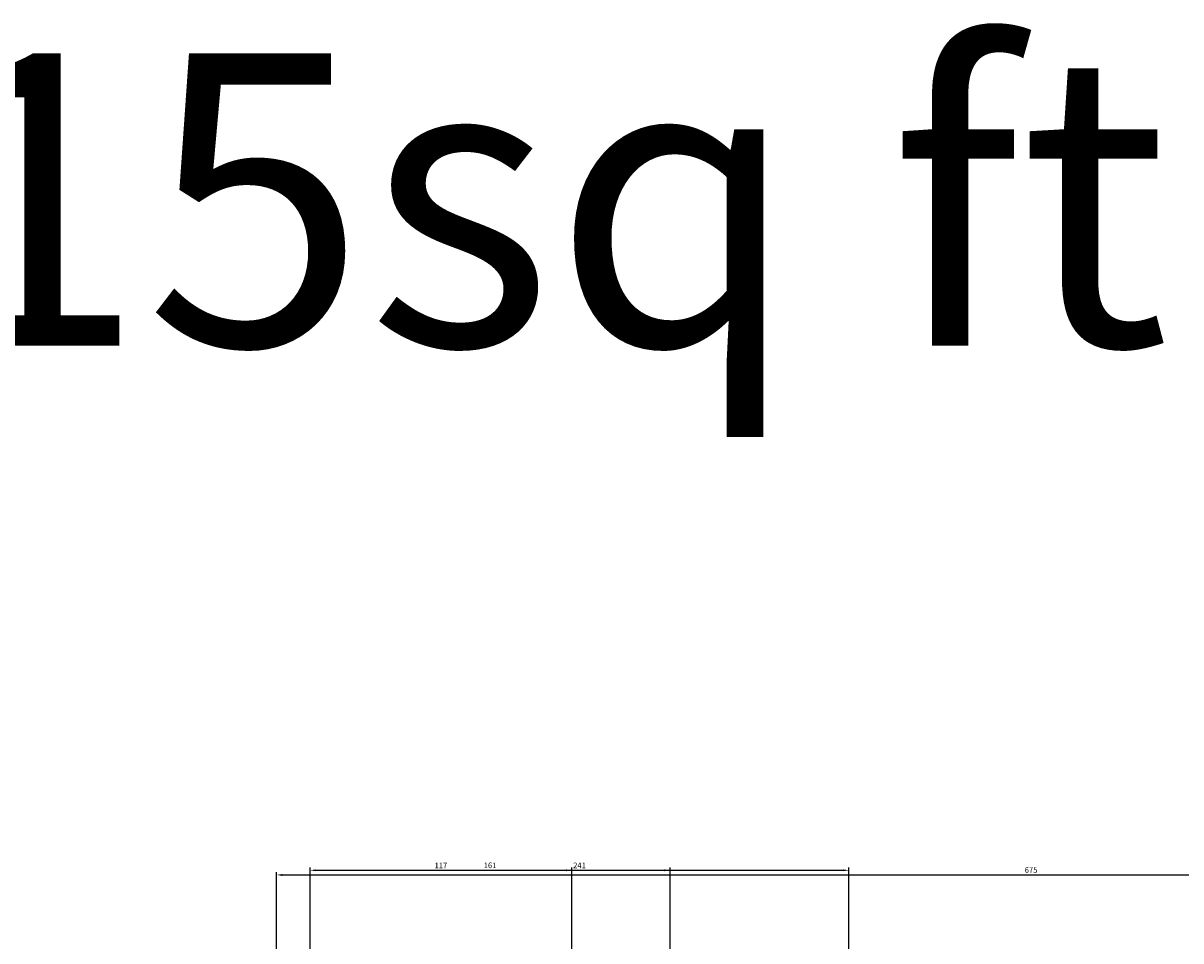
# Model space of a CAD drawing. Units: inches. Extents: x 604 to 3492, y -123 to 1737.
# Tile 18 of 20: x 1461 to 1979, y 1327 to 1737. Entities that reach past the tile are written whole.
import ezdxf

# ---------------------------------------------------------------- set-up
doc = ezdxf.new("R2010")
doc.units = ezdxf.units.IN
doc.layers.add('A-ANNO-DIMS', color=2, linetype='Continuous', lineweight=18)
doc.layers.add('A-ANNO-TEXT', color=7, linetype='Continuous', lineweight=35)
doc.styles.get("Standard").update_dxf_attribs({"font": 'arial.ttf'})
doc.dimstyles.new('ISO-25', dxfattribs={"dimtxt": 2.5, "dimasz": 2.5, "dimexe": 1.25, "dimexo": 0.625, "dimtad": 1, "dimtxsty": 'Standard', "dimcen": 2.5, "dimadec": 0, "dimazin": 0, "dimtfac": 1, "dimtmove": 0, "dimatfit": 3, "dimfxl": 1, "dimarcsym": 0})

# ---------------------------------------------------------------- blocks, each defined once
blk = doc.blocks.new('*D71')
at = {"layer": 'A-ANNO-DIMS', "color": 0, "lineweight": -2, "transparency": 16777216}
for p, q in [((1574.57, 1288.33), (1574.57, 1357.82)), ((2249.57, 1288.33), (2249.57, 1357.82)), ((1577.07, 1356.57), (2247.07, 1356.57))]:
    blk.add_line(p, q, dxfattribs=at)
at = {"layer": 'A-ANNO-DIMS', "color": 0, "transparency": 16777216}
for points in [[(1577.07, 1356.98), (1577.07, 1356.15), (1574.57, 1356.57)], [(2247.07, 1356.98), (2247.07, 1356.15), (2249.57, 1356.57)]]:
    blk.add_solid(points, dxfattribs=at)
at = {"layer": 'Defpoints', "color": 0, "transparency": 16777216}
for p in [(2249.57, 1356.57), (1574.57, 1287.7), (2249.57, 1287.7)]:
    blk.add_point(p, dxfattribs=at)
at = {"layer": 'A-ANNO-DIMS', "color": 0, "transparency": 16777216, "insert": (1912.07, 1358.47), "char_height": 2.5, "attachment_point": 5}
blk.add_mtext('675', dxfattribs=at)
blk = doc.blocks.new('*D100')
at = {"layer": 'A-ANNO-DIMS', "color": 0, "lineweight": -2, "transparency": 16777216}
for p, q in [((1589.57, 843.33), (1589.57, 1359.9)), ((1592.07, 1358.65), (1828.07, 1358.65)), ((1830.57, 843.33), (1830.57, 1359.9))]:
    blk.add_line(p, q, dxfattribs=at)
at = {"layer": 'A-ANNO-DIMS', "color": 0, "transparency": 16777216}
for points in [[(1592.07, 1359.07), (1592.07, 1358.23), (1589.57, 1358.65)], [(1828.07, 1359.07), (1828.07, 1358.23), (1830.57, 1358.65)]]:
    blk.add_solid(points, dxfattribs=at)
at = {"layer": 'Defpoints', "color": 0, "transparency": 16777216}
for p in [(1830.57, 1358.65), (1589.57, 842.7), (1830.57, 842.7)]:
    blk.add_point(p, dxfattribs=at)
at = {"layer": 'A-ANNO-DIMS', "color": 0, "transparency": 16777216, "insert": (1710.07, 1360.53), "char_height": 2.5, "attachment_point": 5}
blk.add_mtext('241', dxfattribs=at)
blk = doc.blocks.new('*D108')
at = {"layer": 'A-ANNO-DIMS', "color": 0, "lineweight": -2, "transparency": 16777216}
for p, q in [((1589.57, 303.33), (1589.57, 1359.9)), ((1592.07, 1358.65), (1704.07, 1358.65)), ((1706.57, 303.33), (1706.57, 1359.9))]:
    blk.add_line(p, q, dxfattribs=at)
at = {"layer": 'A-ANNO-DIMS', "color": 0, "transparency": 16777216}
for points in [[(1592.07, 1359.07), (1592.07, 1358.23), (1589.57, 1358.65)], [(1704.07, 1359.07), (1704.07, 1358.23), (1706.57, 1358.65)]]:
    blk.add_solid(points, dxfattribs=at)
at = {"layer": 'Defpoints', "color": 0, "transparency": 16777216}
for p in [(1706.57, 1358.65), (1589.57, 302.7), (1706.57, 302.7)]:
    blk.add_point(p, dxfattribs=at)
at = {"layer": 'A-ANNO-DIMS', "color": 0, "transparency": 16777216, "insert": (1648.07, 1360.53), "char_height": 2.5, "attachment_point": 5}
blk.add_mtext('117', dxfattribs=at)
blk = doc.blocks.new('*D110')
at = {"layer": 'A-ANNO-DIMS', "color": 0, "lineweight": -2, "transparency": 16777216}
for p, q in [((1589.57, 973.33), (1589.57, 1359.9)), ((1592.07, 1358.65), (1748.07, 1358.65)), ((1750.57, 973.33), (1750.57, 1359.9))]:
    blk.add_line(p, q, dxfattribs=at)
at = {"layer": 'A-ANNO-DIMS', "color": 0, "transparency": 16777216}
for points in [[(1592.07, 1359.07), (1592.07, 1358.23), (1589.57, 1358.65)], [(1748.07, 1359.07), (1748.07, 1358.23), (1750.57, 1358.65)]]:
    blk.add_solid(points, dxfattribs=at)
at = {"layer": 'Defpoints', "color": 0, "transparency": 16777216}
for p in [(1750.57, 1358.65), (1589.57, 972.7), (1750.57, 972.7)]:
    blk.add_point(p, dxfattribs=at)
at = {"layer": 'A-ANNO-DIMS', "color": 0, "transparency": 16777216, "insert": (1670.07, 1360.55), "char_height": 2.5, "attachment_point": 5}
blk.add_mtext('161', dxfattribs=at)

msp = doc.modelspace()

# ---------------------------------------------------------------- texts
at = {"layer": 'A-ANNO-TEXT'}
msp.add_text('4bhk  1415sq ft', height=130.709805, dxfattribs=at).set_placement((723.1092, 1593.2028))

# ---------------------------------------------------------------- dimensions: what is measured, and where the dimension line sits
at = {"layer": 'A-ANNO-DIMS'}
for base, p1, p2, picture, middle in [((1750.5743, 1358.6504), (1589.5743, 972.7004), (1750.5743, 972.7004), '*D110', (1670.0743, 1360.5519)), ((1830.5743, 1358.6504), (1589.5743, 842.7004), (1830.5743, 842.7004), '*D100', (1710.0743, 1360.5306)), ((1706.5743, 1358.6504), (1589.5743, 302.7004), (1706.5743, 302.7004), '*D108', (1648.0743, 1360.5306))]:
    dim = msp.add_linear_dim(base=base, p1=p1, p2=p2, dimstyle='ISO-25', override={"dimdec": 0, "dimlfac": 1, "dimrnd": 0, "dimzin": 0, "dimdsep": 46, "dimlunit": 2}, dxfattribs=at)
    dim.commit()
    dim.dimension.update_dxf_attribs({"geometry": picture, "text_midpoint": middle})
dim = msp.add_aligned_dim(p1=(1574.5743, 1287.7004), p2=(2249.5743, 1287.7004), distance=68.8648, dimstyle='ISO-25', override={"dimclrd": 0, "dimclre": 0, "dimclrt": 0}, dxfattribs=at)
dim.commit()
dim.dimension.update_dxf_attribs({"geometry": '*D71', "text_midpoint": (1912.0743, 1358.4667)})

doc.saveas('drawing.dxf')
